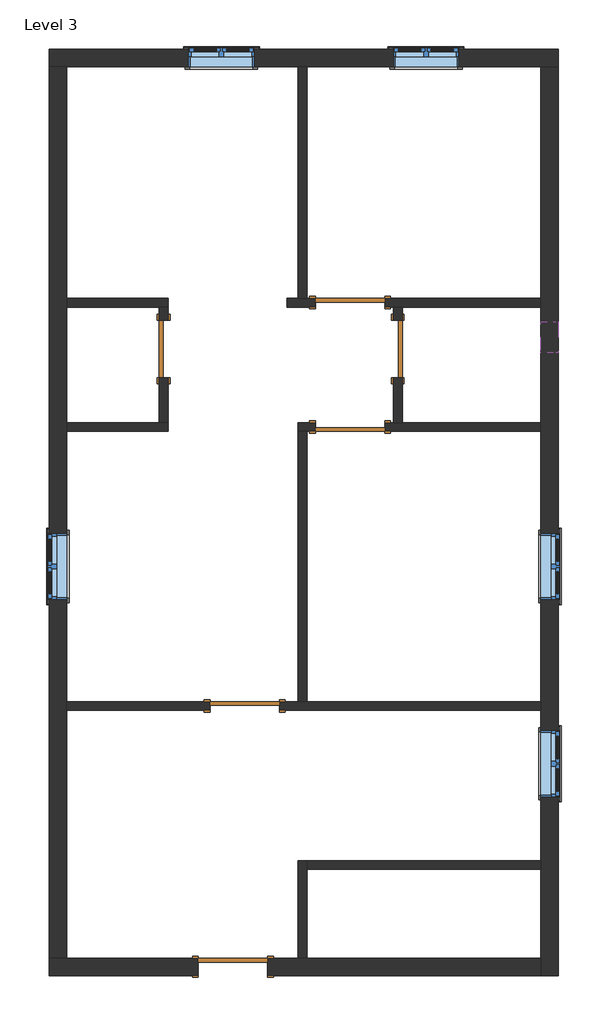
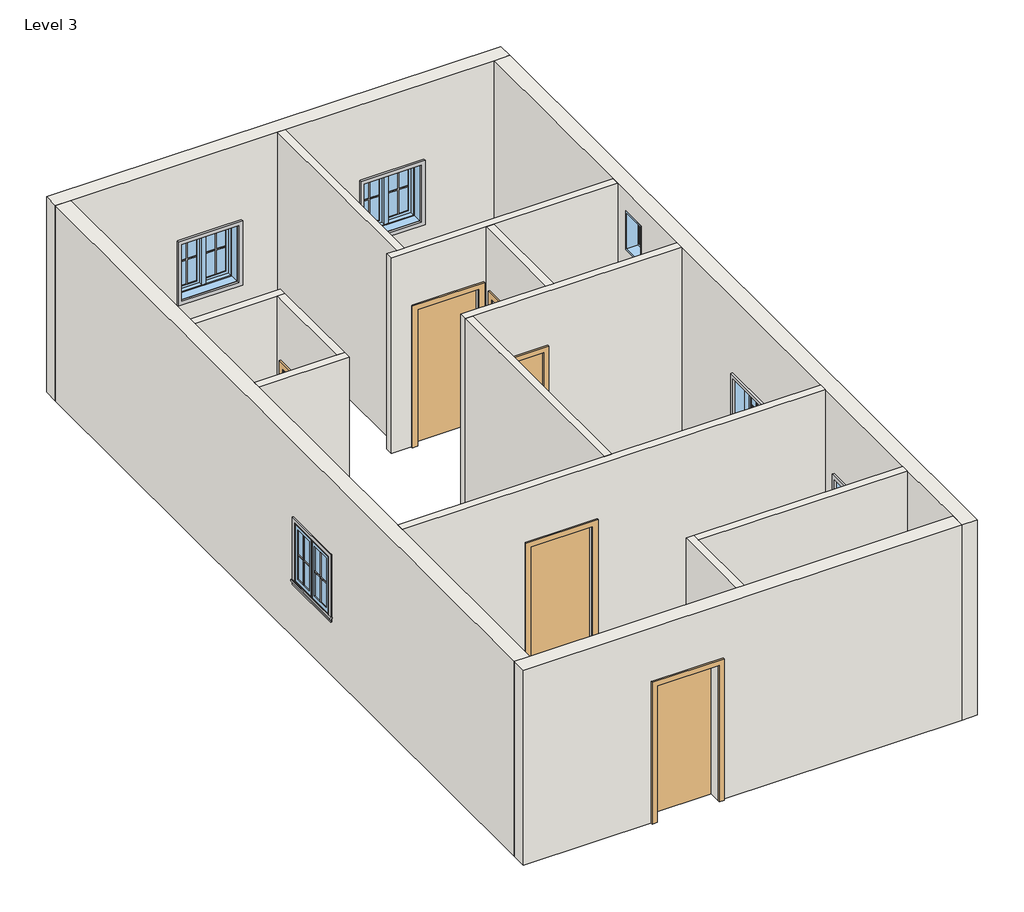
# One storey: 20 proxies, 15 walls, 6 doors, 6 windows.
"""IFC4 building model written with IfcOpenShell, lengths in millimetres."""

from ifc_helpers import new_model, si_unit, frame, origin, place, context, project, spatial, polyline, outline, extrude, faceted_brep, transform, mapped, element, save
from components import muntin_pattern_2x2_muntin_pattern_2x2_b3fe6957, muntin_pattern_2x2_muntin_pattern_2x2_3e0ecaf2, trim_window_exterior_flat_with_sill_41619996, trim_window_interior_flat_picture_frame_51c85655, door_f2b275c1, door_d8f5dbb5, door_305aa2a5, door_e5f9f3c4, door_a90ba1ad, window_aa618e30, window_339605e1

model = new_model("IFC4")

# Units and contexts
model_context = context("Model", 3, world=origin())
ifc_project = project(units=[si_unit("LENGTHUNIT", "METRE", prefix="MILLI")], contexts=[model_context])

# Site, building, storey
site = spatial("IfcSite", under=ifc_project)
building = spatial("IfcBuilding", under=site)
storey = spatial("IfcBuildingStorey", under=building, Name="Level 3", Elevation=3200.4)

# Proxies
placement = place(None, origin())
muntin_pattern_2x2_muntin_pattern_2x2_shape = muntin_pattern_2x2_muntin_pattern_2x2_b3fe6957(model_context)
element("IfcBuildingElementProxy", 1, Name="Muntin Pattern_2x2 : Muntin Pattern_2x2", ObjectType="Muntin Pattern_2x2 : Muntin Pattern_2x2", at=placement, inside=storey, context=model_context, shape_type="MappedRepresentation", body=[
    mapped(muntin_pattern_2x2_muntin_pattern_2x2_shape, transform((-2560.703247, 6624.6685985, 4184.65), x_axis=(1.0, 0.0, 0.0), y_axis=(0.0, 1.0, 0.0), z_axis=(0.0, 0.0, 1.0))),
])
element("IfcBuildingElementProxy", 2, Name="Muntin Pattern_2x2 : Muntin Pattern_2x2", ObjectType="Muntin Pattern_2x2 : Muntin Pattern_2x2", at=placement, inside=storey, context=model_context, shape_type="MappedRepresentation", body=[
    mapped(muntin_pattern_2x2_muntin_pattern_2x2_shape, transform((134.871753, 6624.6685985, 4184.65), x_axis=(1.0, 0.0, 0.0), y_axis=(0.0, 1.0, 0.0), z_axis=(0.0, 0.0, 1.0))),
])
element("IfcBuildingElementProxy", 3, Name="Muntin Pattern_2x2 : Muntin Pattern_2x2", ObjectType="Muntin Pattern_2x2 : Muntin Pattern_2x2", at=placement, inside=storey, context=model_context, shape_type="MappedRepresentation", body=[
    mapped(muntin_pattern_2x2_muntin_pattern_2x2_shape, transform((2082.734253, 41.3060985, 4184.65), x_axis=(0.0, -1.0, 0.0), y_axis=(1.0, 0.0, 0.0), z_axis=(0.0, 0.0, 1.0))),
])
element("IfcBuildingElementProxy", 4, Name="Muntin Pattern_2x2 : Muntin Pattern_2x2", ObjectType="Muntin Pattern_2x2 : Muntin Pattern_2x2", at=placement, inside=storey, context=model_context, shape_type="MappedRepresentation", body=[
    mapped(muntin_pattern_2x2_muntin_pattern_2x2_shape, transform((-4603.815747, -387.3189015, 4184.65), x_axis=(0.0, 1.0, 0.0), y_axis=(-1.0, 0.0, 0.0), z_axis=(0.0, 0.0, 1.0))),
])
element("IfcBuildingElementProxy", 5, Name="Muntin Pattern_2x2 : Muntin Pattern_2x2", ObjectType="Muntin Pattern_2x2 : Muntin Pattern_2x2", at=placement, inside=storey, context=model_context, shape_type="MappedRepresentation", body=[
    mapped(muntin_pattern_2x2_muntin_pattern_2x2_shape, transform((2082.734253, -2555.8439015, 4184.65), x_axis=(0.0, -1.0, 0.0), y_axis=(1.0, 0.0, 0.0), z_axis=(0.0, 0.0, 1.0))),
])
muntin_pattern_2x2_muntin_pattern_2x2_2_shape = muntin_pattern_2x2_muntin_pattern_2x2_3e0ecaf2(model_context)
element("IfcBuildingElementProxy", 6, Name="Muntin Pattern_2x2 : Muntin Pattern_2x2", ObjectType="Muntin Pattern_2x2 : Muntin Pattern_2x2", at=placement, inside=storey, context=model_context, shape_type="MappedRepresentation", body=[
    mapped(muntin_pattern_2x2_muntin_pattern_2x2_2_shape, transform((-2132.078247, 6624.6685985, 4184.65), x_axis=(-1.0, 0.0, 0.0), y_axis=(0.0, -1.0, 0.0), z_axis=(0.0, 0.0, 1.0))),
])
element("IfcBuildingElementProxy", 7, Name="Muntin Pattern_2x2 : Muntin Pattern_2x2", ObjectType="Muntin Pattern_2x2 : Muntin Pattern_2x2", at=placement, inside=storey, context=model_context, shape_type="MappedRepresentation", body=[
    mapped(muntin_pattern_2x2_muntin_pattern_2x2_2_shape, transform((563.496753, 6624.6685985, 4184.65), x_axis=(-1.0, 0.0, 0.0), y_axis=(0.0, -1.0, 0.0), z_axis=(0.0, 0.0, 1.0))),
])
element("IfcBuildingElementProxy", 8, Name="Muntin Pattern_2x2 : Muntin Pattern_2x2", ObjectType="Muntin Pattern_2x2 : Muntin Pattern_2x2", at=placement, inside=storey, context=model_context, shape_type="MappedRepresentation", body=[
    mapped(muntin_pattern_2x2_muntin_pattern_2x2_2_shape, transform((2082.734253, -387.3189015, 4184.65), x_axis=(0.0, 1.0, 0.0), y_axis=(-1.0, 0.0, 0.0), z_axis=(0.0, 0.0, 1.0))),
])
element("IfcBuildingElementProxy", 9, Name="Muntin Pattern_2x2 : Muntin Pattern_2x2", ObjectType="Muntin Pattern_2x2 : Muntin Pattern_2x2", at=placement, inside=storey, context=model_context, shape_type="MappedRepresentation", body=[
    mapped(muntin_pattern_2x2_muntin_pattern_2x2_2_shape, transform((-4603.815747, 41.3060985, 4184.65), x_axis=(0.0, -1.0, 0.0), y_axis=(1.0, 0.0, 0.0), z_axis=(0.0, 0.0, 1.0))),
])
element("IfcBuildingElementProxy", 10, Name="Muntin Pattern_2x2 : Muntin Pattern_2x2", ObjectType="Muntin Pattern_2x2 : Muntin Pattern_2x2", at=placement, inside=storey, context=model_context, shape_type="MappedRepresentation", body=[
    mapped(muntin_pattern_2x2_muntin_pattern_2x2_2_shape, transform((2082.734253, -2984.4689015, 4184.65), x_axis=(0.0, 1.0, 0.0), y_axis=(-1.0, 0.0, 0.0), z_axis=(0.0, 0.0, 1.0))),
])
trim_window_exterior_flat_with_sill_shape = trim_window_exterior_flat_with_sill_41619996(model_context)
element("IfcBuildingElementProxy", 11, Name="Trim-Window-Exterior-Flat : with Sill", ObjectType="Trim-Window-Exterior-Flat : with Sill", at=placement, inside=storey, context=model_context, shape_type="MappedRepresentation", body=[
    mapped(trim_window_exterior_flat_with_sill_shape, transform((-2346.390747, 6634.1935985, 5029.2), x_axis=(-1.0, 0.0, 0.0), y_axis=(0.0, 0.0, 1.0), z_axis=(0.0, 1.0, 0.0))),
])
element("IfcBuildingElementProxy", 12, Name="Trim-Window-Exterior-Flat : with Sill", ObjectType="Trim-Window-Exterior-Flat : with Sill", at=placement, inside=storey, context=model_context, shape_type="MappedRepresentation", body=[
    mapped(trim_window_exterior_flat_with_sill_shape, transform((349.184253, 6634.1935985, 5029.2), x_axis=(-1.0, 0.0, 0.0), y_axis=(0.0, 0.0, 1.0), z_axis=(0.0, 1.0, 0.0))),
])
element("IfcBuildingElementProxy", 13, Name="Trim-Window-Exterior-Flat : with Sill", ObjectType="Trim-Window-Exterior-Flat : with Sill", at=placement, inside=storey, context=model_context, shape_type="MappedRepresentation", body=[
    mapped(trim_window_exterior_flat_with_sill_shape, transform((2092.259253, -173.0064015, 5029.2), x_axis=(0.0, 1.0, 0.0), y_axis=(0.0, 0.0, 1.0), z_axis=(1.0, 0.0, 0.0))),
])
element("IfcBuildingElementProxy", 14, Name="Trim-Window-Exterior-Flat : with Sill", ObjectType="Trim-Window-Exterior-Flat : with Sill", at=placement, inside=storey, context=model_context, shape_type="MappedRepresentation", body=[
    mapped(trim_window_exterior_flat_with_sill_shape, transform((-4613.340747, -173.0064015, 5029.2), x_axis=(0.0, -1.0, 0.0), y_axis=(0.0, 0.0, 1.0), z_axis=(-1.0, 0.0, 0.0))),
])
element("IfcBuildingElementProxy", 15, Name="Trim-Window-Exterior-Flat : with Sill", ObjectType="Trim-Window-Exterior-Flat : with Sill", at=placement, inside=storey, context=model_context, shape_type="MappedRepresentation", body=[
    mapped(trim_window_exterior_flat_with_sill_shape, transform((2092.259253, -2770.1564015, 5029.2), x_axis=(0.0, 1.0, 0.0), y_axis=(0.0, 0.0, 1.0), z_axis=(1.0, 0.0, 0.0))),
])
trim_window_interior_flat_picture_frame_shape = trim_window_interior_flat_picture_frame_51c85655(model_context)
element("IfcBuildingElementProxy", 16, Name="Trim-Window-Interior-Flat : Picture Frame", ObjectType="Trim-Window-Interior-Flat : Picture Frame", at=placement, inside=storey, context=model_context, shape_type="MappedRepresentation", body=[
    mapped(trim_window_interior_flat_picture_frame_shape, transform((-2346.390747, 6405.5935985, 5029.2), x_axis=(1.0, 0.0, 0.0), y_axis=(0.0, 0.0, 1.0), z_axis=(0.0, -1.0, 0.0))),
])
element("IfcBuildingElementProxy", 17, Name="Trim-Window-Interior-Flat : Picture Frame", ObjectType="Trim-Window-Interior-Flat : Picture Frame", at=placement, inside=storey, context=model_context, shape_type="MappedRepresentation", body=[
    mapped(trim_window_interior_flat_picture_frame_shape, transform((349.184253, 6405.5935985, 5029.2), x_axis=(1.0, 0.0, 0.0), y_axis=(0.0, 0.0, 1.0), z_axis=(0.0, -1.0, 0.0))),
])
element("IfcBuildingElementProxy", 18, Name="Trim-Window-Interior-Flat : Picture Frame", ObjectType="Trim-Window-Interior-Flat : Picture Frame", at=placement, inside=storey, context=model_context, shape_type="MappedRepresentation", body=[
    mapped(trim_window_interior_flat_picture_frame_shape, transform((1863.659253, -173.0064015, 5029.2), x_axis=(0.0, -1.0, 0.0), y_axis=(0.0, 0.0, 1.0), z_axis=(-1.0, 0.0, 0.0))),
])
element("IfcBuildingElementProxy", 19, Name="Trim-Window-Interior-Flat : Picture Frame", ObjectType="Trim-Window-Interior-Flat : Picture Frame", at=placement, inside=storey, context=model_context, shape_type="MappedRepresentation", body=[
    mapped(trim_window_interior_flat_picture_frame_shape, transform((-4384.740747, -173.0064015, 5029.2), x_axis=(0.0, 1.0, 0.0), y_axis=(0.0, 0.0, 1.0), z_axis=(1.0, 0.0, 0.0))),
])
element("IfcBuildingElementProxy", 20, Name="Trim-Window-Interior-Flat : Picture Frame", ObjectType="Trim-Window-Interior-Flat : Picture Frame", at=placement, inside=storey, context=model_context, shape_type="MappedRepresentation", body=[
    mapped(trim_window_interior_flat_picture_frame_shape, transform((1863.659253, -2770.1564015, 5029.2), x_axis=(0.0, -1.0, 0.0), y_axis=(0.0, 0.0, 1.0), z_axis=(-1.0, 0.0, 0.0))),
])

# Doors
door_shape = door_f2b275c1(model_context)
element("IfcDoor", 21, ObjectType="Single-Flush : 30\" x 80\"", at=placement, inside=storey, context=model_context, shape_type="MappedRepresentation", body=[
    mapped(door_shape, transform((-22.290747, 2690.8435985, 3200.4), x_axis=(0.0, 1.0, 0.0), y_axis=(-1.0, 0.0, 0.0), z_axis=(0.0, 0.0, 1.0))),
])
door_2_shape = door_d8f5dbb5(model_context)
element("IfcDoor", 22, ObjectType="Single-Flush : 30\" x 80\"", at=placement, inside=storey, context=model_context, shape_type="MappedRepresentation", body=[
    mapped(door_2_shape, transform((-3108.390747, 2690.8435985, 3200.4), x_axis=(0.0, 1.0, 0.0), y_axis=(-1.0, 0.0, 0.0), z_axis=(0.0, 0.0, 1.0))),
])
door_3_shape = door_305aa2a5(model_context)
element("IfcDoor", 23, ObjectType="Single-Flush : 36\" x 84\"", at=placement, inside=storey, context=model_context, shape_type="MappedRepresentation", body=[
    mapped(door_3_shape, transform((-650.940747, 3300.4435985, 3200.4), x_axis=(-1.0, 0.0, 0.0), y_axis=(0.0, -1.0, 0.0), z_axis=(0.0, 0.0, 1.0))),
])
door_4_shape = door_e5f9f3c4(model_context)
element("IfcDoor", 24, ObjectType="Single-Flush : 36\" x 84\"", at=placement, inside=storey, context=model_context, shape_type="MappedRepresentation", body=[
    mapped(door_4_shape, transform((-2041.590747, -2008.1564015, 3200.4), x_axis=(1.0, 0.0, 0.0), y_axis=(0.0, 1.0, 0.0), z_axis=(0.0, 0.0, 1.0))),
])
element("IfcDoor", 25, ObjectType="Single-Flush : 36\" x 84\"", at=placement, inside=storey, context=model_context, shape_type="MappedRepresentation", body=[
    mapped(door_4_shape, transform((-650.940747, 1662.1435985, 3200.4), x_axis=(-1.0, 0.0, 0.0), y_axis=(0.0, -1.0, 0.0), z_axis=(0.0, 0.0, 1.0))),
])
door_5_shape = door_a90ba1ad(model_context)
element("IfcDoor", 26, ObjectType="Single-Flush : 36\" x 84\"", at=placement, inside=storey, context=model_context, shape_type="MappedRepresentation", body=[
    mapped(door_5_shape, transform((-2193.990747, -5443.5064015, 3200.4), x_axis=(-1.0, 0.0, 0.0), y_axis=(0.0, -1.0, 0.0), z_axis=(0.0, 0.0, 1.0))),
])

# Walls
element("IfcWall", 27, ObjectType="WALL4.5\"", at=placement, inside=storey, context=model_context, shape_type="Brep", body=[
    faceted_brep([(-4384.740747, 3243.2935985, 3200.4), (-3165.540747, 3243.2935985, 3200.4), (-3051.240747, 3243.2935985, 3200.4), (-3051.240747, 3243.2935985, 6248.4), (-3165.540747, 3243.2935985, 6248.4), (-4384.740747, 3243.2935985, 6248.4), (-4384.740747, 3357.5935985, 3200.4), (-4384.740747, 3357.5935985, 6248.4), (-3051.240747, 3357.5935985, 6248.4), (-3051.240747, 3357.5935985, 3200.4)], [[[0, 1, 2, 3, 4, 5]], [[6, 7, 8, 9]], [[2, 1, 0, 6, 9]], [[0, 5, 7, 6]], [[3, 2, 9, 8]], [[5, 4, 3, 8, 7]]]),
])
element("IfcWall", 28, ObjectType="WALL4.5\"", at=placement, inside=storey, context=model_context, shape_type="Brep", body=[
    faceted_brep([(-4384.740747, 1604.9935985, 3200.4), (-3051.240747, 1604.9935985, 3200.4), (-3051.240747, 1604.9935985, 6248.4), (-4384.740747, 1604.9935985, 6248.4), (-4384.740747, 1719.2935985, 3200.4), (-4384.740747, 1719.2935985, 6248.4), (-3165.540747, 1719.2935985, 6248.4), (-3051.240747, 1719.2935985, 6248.4), (-3051.240747, 1719.2935985, 3200.4), (-3165.540747, 1719.2935985, 3200.4)], [[[0, 1, 2, 3]], [[4, 5, 6, 7, 8, 9]], [[1, 0, 4, 9, 8]], [[0, 3, 5, 4]], [[2, 1, 8, 7]], [[3, 2, 7, 6, 5]]]),
])
element("IfcWall", 29, ObjectType="WALL4.5\"", at=placement, inside=storey, context=model_context, shape_type="SweptSolid", body=[
    extrude(outline(polyline([(3243.2935985, 3200.4), (3071.8435985, 3200.4), (3071.8435985, 5232.4), (2309.8435985, 5232.4), (2309.8435985, 3200.4), (1719.2935985, 3200.4), (1719.2935985, 6248.4), (3243.2935985, 6248.4), (3243.2935985, 3200.4)])), frame((-3165.540747, 0.0, 0.0), z_axis=(1.0, 0.0, 0.0), x_axis=(0.0, 1.0, 0.0)), (0.0, 0.0, 1.0), 114.3),
])
element("IfcWall", 30, ObjectType="WALL4.5\"", at=placement, inside=storey, context=model_context, shape_type="SweptSolid", body=[
    extrude(outline(polyline([(-1336.740747, 3357.5935985), (-1336.740747, 6405.5935985), (-1222.440747, 6405.5935985), (-1222.440747, 3357.5935985), (-1336.740747, 3357.5935985)])), frame((0.0, 0.0, 3200.4), z_axis=(0.0, 0.0, 1.0), x_axis=(1.0, 0.0, 0.0)), (0.0, 0.0, 1.0), 3048.0),
])
element("IfcWall", 31, ObjectType="WALL4.5\"", at=placement, inside=storey, context=model_context, shape_type="Brep", body=[
    faceted_brep([(-1481.7019184, 3243.2935985, 3200.4), (-1108.140747, 3243.2935985, 3200.4), (-1108.140747, 3243.2935985, 5334.0), (-193.740747, 3243.2935985, 5334.0), (-193.740747, 3243.2935985, 3200.4), (-79.440747, 3243.2935985, 3200.4), (34.859253, 3243.2935985, 3200.4), (1863.659253, 3243.2935985, 3200.4), (1863.659253, 3243.2935985, 6248.4), (34.859253, 3243.2935985, 6248.4), (-79.440747, 3243.2935985, 6248.4), (-1481.7019184, 3243.2935985, 6248.4), (-1108.140747, 3357.5935985, 5334.0), (-1108.140747, 3357.5935985, 3200.4), (-1222.440747, 3357.5935985, 3200.4), (-1336.740747, 3357.5935985, 3200.4), (-1481.7019184, 3357.5935985, 3200.4), (-1481.7019184, 3357.5935985, 6248.4), (-1336.740747, 3357.5935985, 6248.4), (-1222.440747, 3357.5935985, 6248.4), (1863.659253, 3357.5935985, 6248.4), (1863.659253, 3357.5935985, 3200.4), (-193.740747, 3357.5935985, 3200.4), (-193.740747, 3357.5935985, 5334.0)], [[[0, 1, 2, 3, 4, 5, 6, 7, 8, 9, 10, 11]], [[12, 13, 14, 15, 16, 17, 18, 19, 20, 21, 22, 23]], [[22, 21, 7, 6, 5, 4]], [[16, 15, 14, 13, 1, 0]], [[0, 11, 17, 16]], [[8, 7, 21, 20]], [[2, 1, 13, 12]], [[3, 2, 12, 23]], [[4, 3, 23, 22]], [[11, 10, 9, 8, 20, 19, 18, 17]]]),
])
element("IfcWall", 32, ObjectType="WALL4.5\"", at=placement, inside=storey, context=model_context, shape_type="SweptSolid", body=[
    extrude(outline(polyline([(3243.2935985, 3200.4), (3071.8435985, 3200.4), (3071.8435985, 5232.4), (2309.8435985, 5232.4), (2309.8435985, 3200.4), (1719.2935985, 3200.4), (1719.2935985, 6248.4), (3243.2935985, 6248.4), (3243.2935985, 3200.4)])), frame((-79.440747, 0.0, 0.0), z_axis=(1.0, 0.0, 0.0), x_axis=(0.0, 1.0, 0.0)), (0.0, 0.0, 1.0), 114.3),
])
element("IfcWall", 33, ObjectType="WALL4.5\"", at=placement, inside=storey, context=model_context, shape_type="Brep", body=[
    faceted_brep([(-1108.140747, 1719.2935985, 5334.0), (-1108.140747, 1719.2935985, 3200.4), (-1336.740747, 1719.2935985, 3200.4), (-1336.740747, 1719.2935985, 6248.4), (-79.440747, 1719.2935985, 6248.4), (34.859253, 1719.2935985, 6248.4), (1863.659253, 1719.2935985, 6248.4), (1863.659253, 1719.2935985, 3200.4), (34.859253, 1719.2935985, 3200.4), (-79.440747, 1719.2935985, 3200.4), (-193.740747, 1719.2935985, 3200.4), (-193.740747, 1719.2935985, 5334.0), (-1336.740747, 1604.9935985, 3200.4), (-1222.440747, 1604.9935985, 3200.4), (-1108.140747, 1604.9935985, 3200.4), (-1108.140747, 1604.9935985, 5334.0), (-193.740747, 1604.9935985, 5334.0), (-193.740747, 1604.9935985, 3200.4), (1863.659253, 1604.9935985, 3200.4), (1863.659253, 1604.9935985, 6248.4), (-1222.440747, 1604.9935985, 6248.4), (-1336.740747, 1604.9935985, 6248.4)], [[[0, 1, 2, 3, 4, 5, 6, 7, 8, 9, 10, 11]], [[12, 13, 14, 15, 16, 17, 18, 19, 20, 21]], [[2, 1, 14, 13, 12]], [[10, 9, 8, 7, 18, 17]], [[7, 6, 19, 18]], [[3, 2, 12, 21]], [[15, 14, 1, 0]], [[16, 15, 0, 11]], [[17, 16, 11, 10]], [[6, 5, 4, 3, 21, 20, 19]]]),
])
element("IfcWall", 34, ObjectType="WALL4.5\"", at=placement, inside=storey, context=model_context, shape_type="SweptSolid", body=[
    extrude(outline(polyline([(-1336.740747, -1951.0064015), (-1336.740747, 1604.9935985), (-1222.440747, 1604.9935985), (-1222.440747, -1951.0064015), (-1336.740747, -1951.0064015)])), frame((0.0, 0.0, 3200.4), z_axis=(0.0, 0.0, 1.0), x_axis=(1.0, 0.0, 0.0)), (0.0, 0.0, 1.0), 3048.0),
])
element("IfcWall", 35, ObjectType="WALL4.5\"", at=placement, inside=storey, context=model_context, shape_type="Brep", body=[
    faceted_brep([(-1584.390747, -2065.3064015, 5334.0), (-1584.390747, -2065.3064015, 3200.4), (1863.659253, -2065.3064015, 3200.4), (1863.659253, -2065.3064015, 6248.4), (-4384.740747, -2065.3064015, 6248.4), (-4384.740747, -2065.3064015, 3200.4), (-2498.790747, -2065.3064015, 3200.4), (-2498.790747, -2065.3064015, 5334.0), (1863.659253, -1951.0064015, 3200.4), (-1222.440747, -1951.0064015, 3200.4), (-1336.740747, -1951.0064015, 3200.4), (-1584.390747, -1951.0064015, 3200.4), (-1584.390747, -1951.0064015, 5334.0), (-2498.790747, -1951.0064015, 5334.0), (-2498.790747, -1951.0064015, 3200.4), (-4384.740747, -1951.0064015, 3200.4), (-4384.740747, -1951.0064015, 6248.4), (-1336.740747, -1951.0064015, 6248.4), (-1222.440747, -1951.0064015, 6248.4), (1863.659253, -1951.0064015, 6248.4)], [[[0, 1, 2, 3, 4, 5, 6, 7]], [[8, 9, 10, 11, 12, 13, 14, 15, 16, 17, 18, 19]], [[6, 5, 15, 14]], [[2, 1, 11, 10, 9, 8]], [[3, 2, 8, 19]], [[5, 4, 16, 15]], [[12, 11, 1, 0]], [[13, 12, 0, 7]], [[14, 13, 7, 6]], [[4, 3, 19, 18, 17, 16]]]),
])
element("IfcWall", 36, ObjectType="WALL4.5\"", at=placement, inside=storey, context=model_context, shape_type="Brep", body=[
    faceted_brep([(-1222.440747, -5329.2064015, 3200.4), (-1222.440747, -4160.8064015, 3200.4), (-1222.440747, -4046.5064015, 3200.4), (-1222.440747, -4046.5064015, 6248.4), (-1222.440747, -4160.8064015, 6248.4), (-1222.440747, -5329.2064015, 6248.4), (-1336.740747, -5329.2064015, 3200.4), (-1336.740747, -5329.2064015, 6248.4), (-1336.740747, -4046.5064015, 6248.4), (-1336.740747, -4046.5064015, 3200.4)], [[[0, 1, 2, 3, 4, 5]], [[6, 7, 8, 9]], [[2, 1, 0, 6, 9]], [[0, 5, 7, 6]], [[3, 2, 9, 8]], [[5, 4, 3, 8, 7]]]),
])
element("IfcWall", 37, ObjectType="WALL4.5\"", at=placement, inside=storey, context=model_context, shape_type="SweptSolid", body=[
    extrude(outline(polyline([(1863.659253, -4160.8064015), (-1222.440747, -4160.8064015), (-1222.440747, -4046.5064015), (1863.659253, -4046.5064015), (1863.659253, -4160.8064015)])), frame((0.0, 0.0, 3200.4), z_axis=(0.0, 0.0, 1.0), x_axis=(1.0, 0.0, 0.0)), (0.0, 0.0, 1.0), 3048.0),
])
element("IfcWall", 38, ObjectType="WALL9\"", at=placement, inside=storey, context=model_context, shape_type="Brep", body=[
    faceted_brep([(-4613.340747, 6405.5935985, 3200.4), (-4384.740747, 6405.5935985, 3200.4), (-1336.740747, 6405.5935985, 3200.4), (-1222.440747, 6405.5935985, 3200.4), (1863.659253, 6405.5935985, 3200.4), (2092.259253, 6405.5935985, 3200.4), (2092.259253, 6405.5935985, 6248.4), (1863.659253, 6405.5935985, 6248.4), (-1222.440747, 6405.5935985, 6248.4), (-1336.740747, 6405.5935985, 6248.4), (-4384.740747, 6405.5935985, 6248.4), (-4613.340747, 6405.5935985, 6248.4), (-1914.590747, 6405.5935985, 5029.2), (-1914.590747, 6405.5935985, 4114.8), (-2778.190747, 6405.5935985, 4114.8), (-2778.190747, 6405.5935985, 5029.2), (780.984253, 6405.5935985, 5029.2), (780.984253, 6405.5935985, 4114.8), (-82.615747, 6405.5935985, 4114.8), (-82.615747, 6405.5935985, 5029.2), (-4613.340747, 6634.1935985, 3200.4), (-4613.340747, 6634.1935985, 6248.4), (2092.259253, 6634.1935985, 6248.4), (2092.259253, 6634.1935985, 3200.4), (-1914.590747, 6634.1935985, 5029.2), (-2778.190747, 6634.1935985, 5029.2), (-2778.190747, 6634.1935985, 4114.8), (-1914.590747, 6634.1935985, 4114.8), (780.984253, 6634.1935985, 5029.2), (-82.615747, 6634.1935985, 5029.2), (-82.615747, 6634.1935985, 4114.8), (780.984253, 6634.1935985, 4114.8)], [[[0, 1, 2, 3, 4, 5, 6, 7, 8, 9, 10, 11], [12, 13, 14, 15], [16, 17, 18, 19]], [[20, 21, 22, 23], [24, 25, 26, 27], [28, 29, 30, 31]], [[5, 4, 3, 2, 1, 0, 20, 23]], [[6, 5, 23, 22]], [[0, 11, 21, 20]], [[13, 12, 24, 27]], [[14, 13, 27, 26]], [[15, 14, 26, 25]], [[12, 15, 25, 24]], [[17, 16, 28, 31]], [[18, 17, 31, 30]], [[19, 18, 30, 29]], [[16, 19, 29, 28]], [[11, 10, 9, 8, 7, 6, 22, 21]]]),
])
element("IfcWall", 39, ObjectType="WALL9\"", at=placement, inside=storey, context=model_context, shape_type="Brep", body=[
    faceted_brep([(1863.659253, 6405.5935985, 3200.4), (1863.659253, 3357.5935985, 3200.4), (1863.659253, 3243.2935985, 3200.4), (1863.659253, 1719.2935985, 3200.4), (1863.659253, 1604.9935985, 3200.4), (1863.659253, -1951.0064015, 3200.4), (1863.659253, -2065.3064015, 3200.4), (1863.659253, -4046.5064015, 3200.4), (1863.659253, -4160.8064015, 3200.4), (1863.659253, -5329.2064015, 3200.4), (1863.659253, -5557.8064015, 3200.4), (1863.659253, -5557.8064015, 6248.4), (1863.659253, -5329.2064015, 6248.4), (1863.659253, -4160.8064015, 6248.4), (1863.659253, -4046.5064015, 6248.4), (1863.659253, -2065.3064015, 6248.4), (1863.659253, -1951.0064015, 6248.4), (1863.659253, 1604.9935985, 6248.4), (1863.659253, 1719.2935985, 6248.4), (1863.659253, 3243.2935985, 6248.4), (1863.659253, 3357.5935985, 6248.4), (1863.659253, 6405.5935985, 6248.4), (1863.659253, 2640.0435985, 5943.6), (1863.659253, 2640.0435985, 5334.0), (1863.659253, 3046.4435985, 5334.0), (1863.659253, 3046.4435985, 5943.6), (1863.659253, -604.8064015, 5029.2), (1863.659253, -604.8064015, 4114.8), (1863.659253, 258.7935985, 4114.8), (1863.659253, 258.7935985, 5029.2), (1863.659253, -3201.9564015, 5029.2), (1863.659253, -3201.9564015, 4114.8), (1863.659253, -2338.3564015, 4114.8), (1863.659253, -2338.3564015, 5029.2), (2092.259253, 6405.5935985, 3200.4), (2092.259253, 6405.5935985, 6248.4), (2092.259253, -5557.8064015, 6248.4), (2092.259253, -5557.8064015, 3200.4), (2092.259253, 2640.0435985, 5943.6), (2092.259253, 3046.4435985, 5943.6), (2092.259253, 3046.4435985, 5334.0), (2092.259253, 2640.0435985, 5334.0), (2092.259253, -604.8064015, 5029.2), (2092.259253, 258.7935985, 5029.2), (2092.259253, 258.7935985, 4114.8), (2092.259253, -604.8064015, 4114.8), (2092.259253, -3201.9564015, 5029.2), (2092.259253, -2338.3564015, 5029.2), (2092.259253, -2338.3564015, 4114.8), (2092.259253, -3201.9564015, 4114.8)], [[[0, 1, 2, 3, 4, 5, 6, 7, 8, 9, 10, 11, 12, 13, 14, 15, 16, 17, 18, 19, 20, 21], [22, 23, 24, 25], [26, 27, 28, 29], [30, 31, 32, 33]], [[34, 35, 36, 37], [38, 39, 40, 41], [42, 43, 44, 45], [46, 47, 48, 49]], [[10, 9, 8, 7, 6, 5, 4, 3, 2, 1, 0, 34, 37]], [[0, 21, 35, 34]], [[11, 10, 37, 36]], [[23, 22, 38, 41]], [[24, 23, 41, 40]], [[25, 24, 40, 39]], [[22, 25, 39, 38]], [[27, 26, 42, 45]], [[28, 27, 45, 44]], [[29, 28, 44, 43]], [[26, 29, 43, 42]], [[31, 30, 46, 49]], [[32, 31, 49, 48]], [[33, 32, 48, 47]], [[30, 33, 47, 46]], [[21, 20, 19, 18, 17, 16, 15, 14, 13, 12, 11, 36, 35]]]),
])
element("IfcWall", 40, ObjectType="WALL9\"", at=placement, inside=storey, context=model_context, shape_type="Brep", body=[
    faceted_brep([(-2651.190747, -5329.2064015, 5334.0), (-2651.190747, -5329.2064015, 3200.4), (-4384.740747, -5329.2064015, 3200.4), (-4613.340747, -5329.2064015, 3200.4), (-4613.340747, -5329.2064015, 6248.4), (-4384.740747, -5329.2064015, 6248.4), (-1336.740747, -5329.2064015, 6248.4), (-1222.440747, -5329.2064015, 6248.4), (1863.659253, -5329.2064015, 6248.4), (1863.659253, -5329.2064015, 3200.4), (-1222.440747, -5329.2064015, 3200.4), (-1336.740747, -5329.2064015, 3200.4), (-1736.790747, -5329.2064015, 3200.4), (-1736.790747, -5329.2064015, 5334.0), (-4613.340747, -5557.8064015, 3200.4), (-2651.190747, -5557.8064015, 3200.4), (-2651.190747, -5557.8064015, 5334.0), (-1736.790747, -5557.8064015, 5334.0), (-1736.790747, -5557.8064015, 3200.4), (1863.659253, -5557.8064015, 3200.4), (1863.659253, -5557.8064015, 6248.4), (-4613.340747, -5557.8064015, 6248.4)], [[[0, 1, 2, 3, 4, 5, 6, 7, 8, 9, 10, 11, 12, 13]], [[14, 15, 16, 17, 18, 19, 20, 21]], [[3, 2, 1, 15, 14]], [[12, 11, 10, 9, 19, 18]], [[9, 8, 20, 19]], [[4, 3, 14, 21]], [[16, 15, 1, 0]], [[17, 16, 0, 13]], [[18, 17, 13, 12]], [[8, 7, 6, 5, 4, 21, 20]]]),
])
element("IfcWall", 41, ObjectType="WALL9\"", at=placement, inside=storey, context=model_context, shape_type="Brep", body=[
    faceted_brep([(-4384.740747, -5329.2064015, 3200.4), (-4384.740747, -2065.3064015, 3200.4), (-4384.740747, -1951.0064015, 3200.4), (-4384.740747, 1604.9935985, 3200.4), (-4384.740747, 1719.2935985, 3200.4), (-4384.740747, 3243.2935985, 3200.4), (-4384.740747, 3357.5935985, 3200.4), (-4384.740747, 6405.5935985, 3200.4), (-4384.740747, 6405.5935985, 6248.4), (-4384.740747, 3357.5935985, 6248.4), (-4384.740747, 3243.2935985, 6248.4), (-4384.740747, 1719.2935985, 6248.4), (-4384.740747, 1604.9935985, 6248.4), (-4384.740747, -1951.0064015, 6248.4), (-4384.740747, -2065.3064015, 6248.4), (-4384.740747, -5329.2064015, 6248.4), (-4384.740747, 258.7935985, 5029.2), (-4384.740747, 258.7935985, 4114.8), (-4384.740747, -604.8064015, 4114.8), (-4384.740747, -604.8064015, 5029.2), (-4613.340747, -5329.2064015, 3200.4), (-4613.340747, -5329.2064015, 6248.4), (-4613.340747, 6405.5935985, 6248.4), (-4613.340747, 6405.5935985, 3200.4), (-4613.340747, 258.7935985, 5029.2), (-4613.340747, -604.8064015, 5029.2), (-4613.340747, -604.8064015, 4114.8), (-4613.340747, 258.7935985, 4114.8)], [[[0, 1, 2, 3, 4, 5, 6, 7, 8, 9, 10, 11, 12, 13, 14, 15], [16, 17, 18, 19]], [[20, 21, 22, 23], [24, 25, 26, 27]], [[7, 6, 5, 4, 3, 2, 1, 0, 20, 23]], [[8, 7, 23, 22]], [[0, 15, 21, 20]], [[17, 16, 24, 27]], [[18, 17, 27, 26]], [[19, 18, 26, 25]], [[16, 19, 25, 24]], [[15, 14, 13, 12, 11, 10, 9, 8, 22, 21]]]),
])

# Windows
window_shape = window_aa618e30(model_context)
element("IfcWindow", 42, ObjectType="Fixed : 16\" x 24\"", at=placement, inside=storey, context=model_context, shape_type="MappedRepresentation", body=[
    mapped(window_shape, transform((1977.959253, 2805.1435985, 4419.6), x_axis=(0.0, -1.0, 0.0), y_axis=(1.0, 0.0, 0.0), z_axis=(0.0, 0.0, 1.0))),
])
window_2_shape = window_339605e1(model_context)
element("IfcWindow", 43, ObjectType="Window-Casement-Double : 34\" x 36\"", at=placement, inside=storey, context=model_context, shape_type="MappedRepresentation", body=[
    mapped(window_2_shape, transform((-2346.390747, 6519.8935985, 3200.4), x_axis=(1.0, 0.0, 0.0), y_axis=(0.0, 1.0, 0.0), z_axis=(0.0, 0.0, 1.0))),
])
element("IfcWindow", 44, ObjectType="Window-Casement-Double : 34\" x 36\"", at=placement, inside=storey, context=model_context, shape_type="MappedRepresentation", body=[
    mapped(window_2_shape, transform((349.184253, 6519.8935985, 3200.4), x_axis=(1.0, 0.0, 0.0), y_axis=(0.0, 1.0, 0.0), z_axis=(0.0, 0.0, 1.0))),
])
element("IfcWindow", 45, ObjectType="Window-Casement-Double : 34\" x 36\"", at=placement, inside=storey, context=model_context, shape_type="MappedRepresentation", body=[
    mapped(window_2_shape, transform((1977.959253, -173.0064015, 3200.4), x_axis=(0.0, -1.0, 0.0), y_axis=(1.0, 0.0, 0.0), z_axis=(0.0, 0.0, 1.0))),
])
element("IfcWindow", 46, ObjectType="Window-Casement-Double : 34\" x 36\"", at=placement, inside=storey, context=model_context, shape_type="MappedRepresentation", body=[
    mapped(window_2_shape, transform((-4499.040747, -173.0064015, 3200.4), x_axis=(0.0, 1.0, 0.0), y_axis=(-1.0, 0.0, 0.0), z_axis=(0.0, 0.0, 1.0))),
])
element("IfcWindow", 47, ObjectType="Window-Casement-Double : 34\" x 36\"", at=placement, inside=storey, context=model_context, shape_type="MappedRepresentation", body=[
    mapped(window_2_shape, transform((1977.959253, -2770.1564015, 3200.4), x_axis=(0.0, -1.0, 0.0), y_axis=(1.0, 0.0, 0.0), z_axis=(0.0, 0.0, 1.0))),
])

save(model, "model.ifc")

# Revit data of these elements
# Type "Muntin Pattern_2x2 : Muntin Pattern_2x2"
#   Width [instance default] = 4' - 0"
#   Thickness = 0' - 0 1/2"
#   Height [instance default] = 4' - 0"
#   Distance = 0' - 0 3/4"
#   Interior Material [instance default] = none
#   Exterior Material [instance default] = none
#   Default Elevation = 0
# Type "Trim-Window-Exterior-Flat : with Sill"
#   Trim Width = 0' - 2 1/4"
#   Trim Thickness_Picture Frame = 0' - 1 1/4"
#   Trim Thickness_with Sill = 0' - 0 3/4"
#   Sill Thickness = 0' - 1 1/4"
#   Opening Width [instance default] = 2' - 0"
#   Opening Height [instance default] = 3' - 0"
#   Default Elevation = 4' - 0"
#   Sill = yes
#   Picture Frame = no
#   Trim Material [instance default] = none
# Type "Trim-Window-Interior-Flat : Picture Frame"
#   Trim Thickness_Picture Frame = 0' - 1 1/4"
#   Trim Width = 0' - 2 1/4"
#   Trim Thickness_with Sill = 0' - 0 3/4"
#   Sill Thickness = 0' - 1 1/4"
#   Opening Width [instance default] = 2' - 0"
#   Opening Height [instance default] = 3' - 0"
#   Default Elevation = 4' - 0"
#   Sill = no
#   Picture Frame = yes
#   Trim Material [instance default] = none
# Type "Single-Flush : 30\" x 80\""
#   Type Mark = "5"
#   Construction Type Id = "MDOOR"
#   Assembly Code = "C1020"
#   Analytic Construction = "Metal"
#   Thickness = 0' - 2"
#   Heat Transfer Coefficient (U) = 0.651978 BTU/(h·ft²·°F)
#   Height = 6' - 8"
#   Trim Projection Ext = 0' - 1"
#   Trim Projection Int = 0' - 1"
#   Trim Width = 0' - 3"
#   Width = 2' - 6"
#   Define Thermal Properties by = 1
#   Define Thermal Properties by = 1
#   Door Material = Door - Panel
#   Frame Material = Door - Frame
#   Visual Light Transmittance = 0
#   Solar Heat Gain Coefficient = 0
#   Function = (empty or 0)
#   Wall Closure = (empty or 0)
# Type "Single-Flush : 36\" x 84\""
#   Type Mark = "1"
#   Construction Type Id = "MDOOR"
#   Assembly Code = "C1020"
#   Analytic Construction = "Metal"
#   Thickness = 0' - 2"
#   Heat Transfer Coefficient (U) = 0.651978 BTU/(h·ft²·°F)
#   Height = 7' - 0"
#   Trim Projection Ext = 0' - 1"
#   Trim Projection Int = 0' - 1"
#   Trim Width = 0' - 3"
#   Width = 3' - 0"
#   Define Thermal Properties by = 1
#   Define Thermal Properties by = 1
#   Door Material = Door - Panel
#   Frame Material = Door - Frame
#   Visual Light Transmittance = 0
#   Solar Heat Gain Coefficient = 0
#   Function = (empty or 0)
#   Wall Closure = (empty or 0)
# Type "WALL4.5\""
#   Assembly Code = "B2010"
#   Layers, outside or top first: 0' - 4 1/2" no material (function 1)
# Type "WALL9\""
#   Assembly Code = "B2010"
#   Layers, outside or top first: 0' - 9" no material (function 1)
# Type "Fixed : 16\" x 24\""
#   Type Mark = "4"
#   Construction Type Id = "GSP4R"
#   Assembly Code = "B2020100"
#   Analytic Construction = "1/8 in Pilkington single glazing"
#   Visual Light Transmittance = 0.9
#   Solar Heat Gain Coefficient = 0.78
#   Heat Transfer Coefficient (U) = 0.6496 BTU/(h·ft²·°F)
#   Height = 2' - 0"
#   Default Sill Height = 3' - 0"
#   Width = 1' - 4"
#   Window Inset = 0' - 0 3/4"
#   Define Thermal Properties by = 1
#   Define Thermal Properties by = 1
#   Glass Pane Material = Glass
#   Sash Material = Sash
#   Wall Closure = (empty or 0)
# Type "Window-Casement-Double : 34\" x 36\""
#   Type Mark = "14"
#   Fire Rating = "0.5h"
#   Assembly Code = "B2020100"
#   Analytic Construction = "Double glazing - domestic"
#   Frame Extension [instance default] = 0' - 0 1/4"
#   Window Inset [instance default] = 0' - 0"
#   Wall Thickness [instance default] = 0' - 6"
#   Interior Wall Closure [instance default] = 0' - 2 1/4"
#   Half Width = 1' - 5"
#   Visual Light Transmittance = 0.81
#   Thermal Resistance (R) = 1.8146 (h·ft²·°F)/BTU
#   Solar Heat Gain Coefficient = 0.76
#   Rough Width = 2' - 10 1/2"
#   Rough Height = 3' - 0 1/2"
#   Height = 3' - 0"
#   Heat Transfer Coefficient (U) = 0.5511 BTU/(h·ft²·°F)
#   Exterior Wall Closure [instance default] = 0' - 1 1/4"
#   Extension Jamb [instance default] = 0' - 2 1/4"
#   Default Sill Height = 3' - 0"
#   Width = 2' - 10"
#   Define Thermal Properties by = 0
#   Muntin Visibility = yes
#   Interior Trim Visibility [instance default] = yes
#   Exterior Trim Visibility [instance default] = yes
#   Extension Jamb Visibility [instance default] = yes
#   Interior Trim Material = Wood - Stained
#   Muntin Pattern = Muntin Pattern_2x2 : Muntin Pattern_2x2
#   Interior Trim = Trim-Window-Interior-Flat : Picture Frame
#   Interior Frame Material = Wood - Stained
#   Glass Panel Material = Glass
#   Exterior Trim Material = Clad - White
#   Exterior Trim = Trim-Window-Exterior-Flat : with Sill
#   Exterior Frame Material = Clad - White
#   Wall Closure = (empty or 0)
# Elements 1, 2, 3, 4, 5, 6, 7, 8, 9, 10 (IfcBuildingElementProxy, "Muntin Pattern_2x2 : Muntin Pattern_2x2")
#   Width = 0' - 11 5/8"
#   Height = 2' - 6 1/2"
#   Interior Material = Wood - Stained
#   Exterior Material = Clad - White
#   Phase Created = New Construction
#   Materials on its faces: "Clad - White", "Wood - Stained"
# Elements 11, 12, 13, 14, 15 (IfcBuildingElementProxy, "Trim-Window-Exterior-Flat : with Sill")
#   Opening Width = 2' - 10"
#   Opening Height = 3' - 0"
#   Trim Material = Clad - White
#   Phase Created = New Construction
#   Materials on its faces: "Clad - White"
# Elements 16, 17, 18, 19, 20 (IfcBuildingElementProxy, "Trim-Window-Interior-Flat : Picture Frame")
#   Opening Width = 2' - 10"
#   Opening Height = 3' - 0"
#   Trim Material = Wood - Stained
#   Phase Created = New Construction
#   Materials on its faces: "Wood - Stained"
# Elements 21, 22 (IfcDoor, "Single-Flush : 30\" x 80\"")
#   Phase Created = New Construction
#   Materials on its faces: "Door - Frame", "Door - Panel"
# Elements 23, 24, 25, 26 (IfcDoor, "Single-Flush : 36\" x 84\"")
#   Phase Created = New Construction
#   Materials on its faces: "Door - Frame", "Door - Panel"
# Elements 27, 28, 29, 30, 31, 32, 33, 34, 35, 36, 37 (IfcWall, "WALL4.5\"")
#   Top Offset = 0' - 0"
#   Base Offset = 0' - 0"
#   Unconnected Height = 10' - 0"
#   wall height = 10' - 0"
#   Phase Created = New Construction
#   Base Constraint = Level 3
#   Materials on its faces: "Default Wall"
# Elements 38, 39, 40, 41 (IfcWall, "WALL9\"")
#   Top Offset = 0' - 0"
#   Base Offset = 0' - 0"
#   Unconnected Height = 10' - 0"
#   wall height = 10' - 0"
#   Phase Created = New Construction
#   Base Constraint = Level 3
#   Materials on its faces: "Default Wall", "Door - Panel"
# Element 42 (IfcWindow, "Fixed : 16\" x 24\"")
#   Mark = "7"
#   Phase Created = New Construction
#   Materials on its faces: "Sash", "Glass"
# Element 43 (IfcWindow, "Window-Casement-Double : 34\" x 36\"")
#   Mark = "8"
#   Window Inset = 0' - 0"
#   Interior Wall Closure = 0' - 2 1/4"
#   Frame Extension = 0' - 0 1/4"
#   Exterior Wall Closure = 0' - 1 1/4"
#   Interior Trim Visibility = yes
#   Exterior Trim Visibility = yes
#   Phase Created = New Construction
#   Materials on its faces: "Wood - Stained", "Glass", "Clad - White"
# Element 44 (IfcWindow, "Window-Casement-Double : 34\" x 36\"")
#   Mark = "9"
#   Window Inset = 0' - 0"
#   Interior Wall Closure = 0' - 2 1/4"
#   Frame Extension = 0' - 0 1/4"
#   Exterior Wall Closure = 0' - 1 1/4"
#   Interior Trim Visibility = yes
#   Exterior Trim Visibility = yes
#   Phase Created = New Construction
#   Materials on its faces: "Wood - Stained", "Glass", "Clad - White"
# Element 45 (IfcWindow, "Window-Casement-Double : 34\" x 36\"")
#   Mark = "10"
#   Window Inset = 0' - 0"
#   Interior Wall Closure = 0' - 2 1/4"
#   Frame Extension = 0' - 0 1/4"
#   Exterior Wall Closure = 0' - 1 1/4"
#   Interior Trim Visibility = yes
#   Exterior Trim Visibility = yes
#   Phase Created = New Construction
#   Materials on its faces: "Wood - Stained", "Glass", "Clad - White"
# Element 46 (IfcWindow, "Window-Casement-Double : 34\" x 36\"")
#   Mark = "11"
#   Window Inset = 0' - 0"
#   Interior Wall Closure = 0' - 2 1/4"
#   Frame Extension = 0' - 0 1/4"
#   Exterior Wall Closure = 0' - 1 1/4"
#   Interior Trim Visibility = yes
#   Exterior Trim Visibility = yes
#   Phase Created = New Construction
#   Materials on its faces: "Wood - Stained", "Glass", "Clad - White"
# Element 47 (IfcWindow, "Window-Casement-Double : 34\" x 36\"")
#   Mark = "12"
#   Window Inset = 0' - 0"
#   Interior Wall Closure = 0' - 2 1/4"
#   Frame Extension = 0' - 0 1/4"
#   Exterior Wall Closure = 0' - 1 1/4"
#   Interior Trim Visibility = yes
#   Exterior Trim Visibility = yes
#   Phase Created = New Construction
#   Materials on its faces: "Wood - Stained", "Glass", "Clad - White"
# Materials
#   "Door - Panel": class "Wood", colour RGB 210 159 95, transparency 0, Cost = 0
#   "Door - Frame": colour RGB 118 70 51, transparency 0, Cost = 0
#   "Glass": class "Glass", colour RGB 0 128 192, transparency 0.75, Description = "Soda Lime Glass", Cost = 0
#   "Sash": class "Wood", colour RGB 224 178 126, transparency 0, Cost = 0
#   "Wood - Stained": class "Wood", colour RGB 224 178 126, transparency 0, Cost = 0
#   "Clad - White": class "Wood", colour RGB 242 242 238, transparency 0, Cost = 0
#   "Default Wall": colour RGB 128 128 128, transparency 0, Cost = 0
